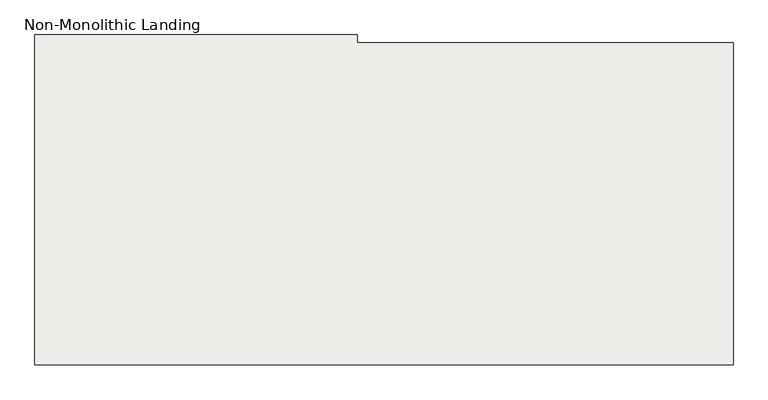
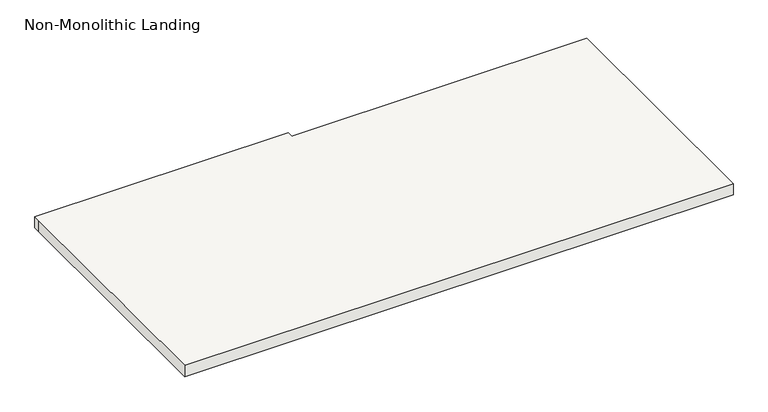
"""IFC4 building model written with IfcOpenShell, lengths in millimetres: slab geometry, Non-Monolithic Landing."""

from ifc_helpers import new_model, si_unit, origin, place, context, project, spatial, faceted_brep, source, transform, mapped, element, save


def non_monolithic_landing_4bbdd230(model_context):
    return source(origin(), model_context, "Body", "Brep", [
        faceted_brep([(-15047.8847893, 9995.9922903, 1435.6772727), (-15047.8847893, 9970.5922903, 1410.2772727), (-16114.6847893, 9970.5922903, 1410.2772727), (-16114.6847893, 9995.9922903, 1435.6772727), (-16292.4847893, 9995.9922903, 1454.7272727), (-16292.4847893, 10021.3922903, 1454.7272727), (-17359.2847893, 10021.3922903, 1454.7272727), (-17359.2847893, 9995.9922903, 1454.7272727), (-17359.2847893, 8929.1922903, 1454.7272727), (-15047.8847893, 8929.1922903, 1454.7272727), (-15047.8847893, 9995.9922903, 1454.7272727), (-16114.6847893, 9970.5922903, 1403.9272727), (-15047.8847893, 9970.5922903, 1403.9272727), (-15047.8847893, 8929.1922903, 1403.9272727), (-17359.2847893, 8929.1922903, 1403.9272727), (-17359.2847893, 9995.9922903, 1403.9272727), (-17359.2847893, 10021.3922903, 1403.9272727), (-16292.4847893, 10021.3922903, 1403.9272727), (-16292.4847893, 9995.9922903, 1403.9272727), (-16114.6847893, 9995.9922903, 1403.9272727)], [[[0, 1, 2, 3]], [[4, 5, 6, 7, 8, 9, 10]], [[11, 12, 13, 14, 15, 16, 17, 18, 19]], [[12, 11, 2, 1]], [[11, 19, 3, 2]], [[4, 10, 0, 3, 19, 18]], [[5, 4, 18, 17]], [[6, 5, 17, 16]], [[7, 6, 16, 15]], [[8, 7, 15, 14]], [[9, 8, 14, 13]], [[10, 9, 13, 12, 1, 0]]]),
    ])


if __name__ == "__main__":
    model = new_model("IFC4")
    model_context = context("Model", 3, world=origin())
    ifc_project = project(units=[si_unit("LENGTHUNIT", "METRE", prefix="MILLI")], contexts=[model_context])
    site = spatial("IfcSite", under=ifc_project)
    building = spatial("IfcBuilding", under=site)
    placement = place(None, origin())
    non_monolithic_landing_shape = non_monolithic_landing_4bbdd230(model_context)
    element("IfcSlab", 1, ObjectType="Non-Monolithic Landing", at=placement, inside=building, context=model_context, shape_type="MappedRepresentation", body=[
        mapped(non_monolithic_landing_shape, transform((0.0, 0.0, 0.0), x_axis=(1.0, 0.0, 0.0), y_axis=(0.0, 1.0, 0.0), z_axis=(0.0, 0.0, 1.0))),
    ])
    save(model, "model.ifc")
